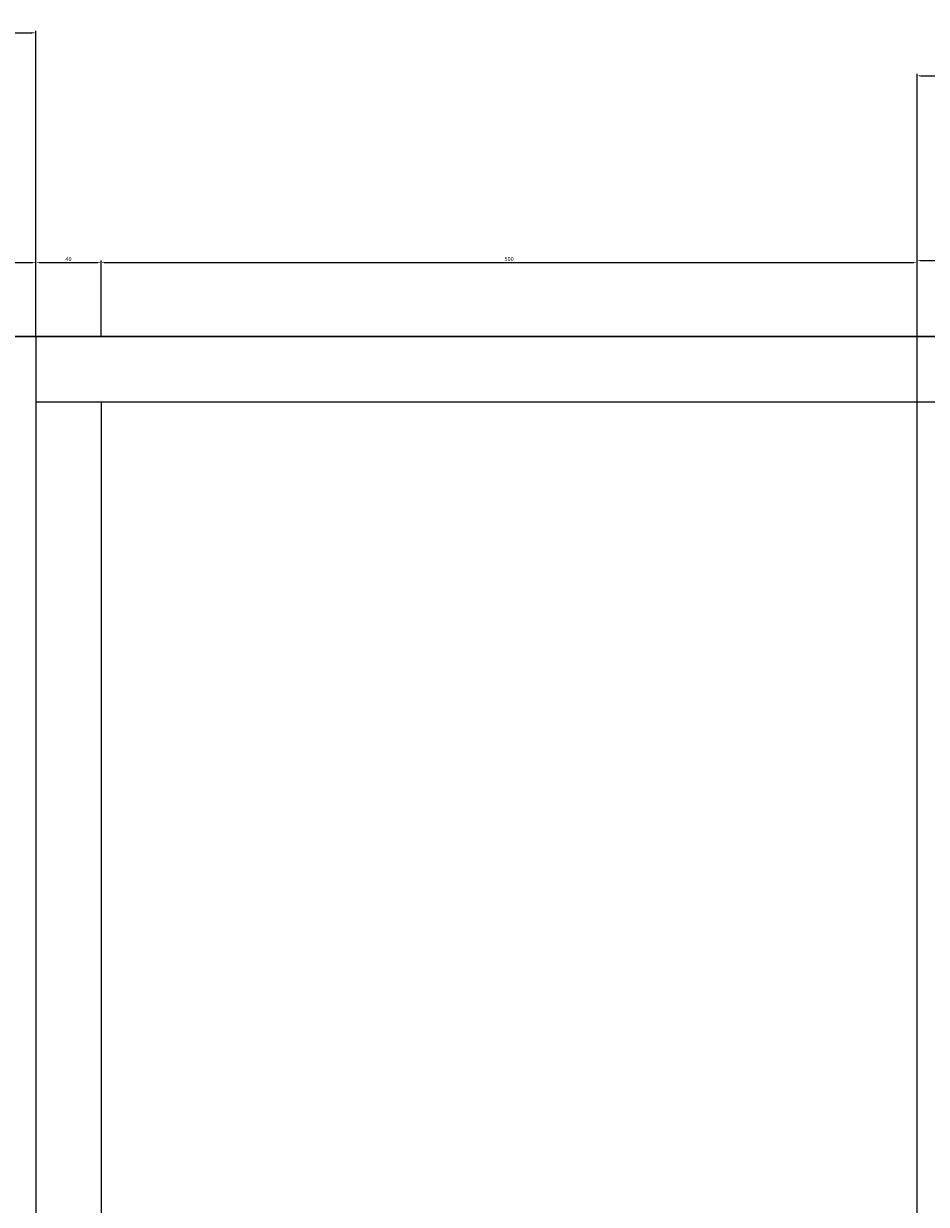
# Model space of a CAD drawing. Units: millimetres. Extents: x 2332 to 5836, y -853 to 2199.
# Tile 6 of 16: x 3088 to 3641, y 1476 to 2199. Entities that reach past the tile are written whole.
import ezdxf

# ---------------------------------------------------------------- set-up
doc = ezdxf.new("R2010")
doc.units = ezdxf.units.MM
doc.layers.get('0').update_dxf_attribs({"color": 8})
for name, color, linetype, lineweight in [('A-ANNO-DIMS', 2, 'Continuous', 18), ('A-WALL', 8, 'Continuous', 30), ('SHELF', 40, 'Continuous', 25)]:
    doc.layers.add(name, color=color, linetype=linetype, lineweight=lineweight)
doc.styles.get("Standard").update_dxf_attribs({"font": 'arial.ttf'})
doc.dimstyles.new('ISO-25', dxfattribs={"dimtxt": 2.5, "dimasz": 2.5, "dimexe": 1.25, "dimexo": 0.625, "dimtad": 1, "dimtxsty": 'Standard', "dimcen": 2.5, "dimadec": 0, "dimazin": 0, "dimtfac": 1, "dimtmove": 0, "dimatfit": 3, "dimfxl": 1, "dimarcsym": 0})

# ---------------------------------------------------------------- blocks, each defined once
blk = doc.blocks.new('*D1')
at = {"layer": 'A-ANNO-DIMS', "color": 0, "lineweight": -2, "transparency": 16777216}
for p, q in [((2745.04, 2008.43), (2745.04, 2054.25)), ((3095.04, 2008.43), (3095.04, 2054.25)), ((2747.54, 2053), (3092.54, 2053))]:
    blk.add_line(p, q, dxfattribs=at)
at = {"layer": 'A-ANNO-DIMS', "color": 0, "transparency": 16777216}
for points in [[(2747.54, 2053.41), (2747.54, 2052.58), (2745.04, 2053)], [(3092.54, 2053.41), (3092.54, 2052.58), (3095.04, 2053)]]:
    blk.add_solid(points, dxfattribs=at)
at = {"layer": 'Defpoints', "color": 0, "transparency": 16777216}
for p in [(3095.04, 2053), (2745.04, 2007.8), (3095.04, 2007.8)]:
    blk.add_point(p, dxfattribs=at)
at = {"layer": 'A-ANNO-DIMS', "color": 0, "transparency": 16777216, "insert": (2920.04, 2054.9), "char_height": 2.5, "attachment_point": 5}
blk.add_mtext('350', dxfattribs=at)
blk = doc.blocks.new('*D2')
at = {"layer": 'A-ANNO-DIMS', "color": 0, "lineweight": -2, "transparency": 16777216}
for p, q in [((3095.04, 2008.43), (3095.04, 2054.25)), ((3135.04, 2008.43), (3135.04, 2054.25)), ((3097.54, 2053), (3132.54, 2053))]:
    blk.add_line(p, q, dxfattribs=at)
at = {"layer": 'A-ANNO-DIMS', "color": 0, "transparency": 16777216}
for points in [[(3097.54, 2053.41), (3097.54, 2052.58), (3095.04, 2053)], [(3132.54, 2053.41), (3132.54, 2052.58), (3135.04, 2053)]]:
    blk.add_solid(points, dxfattribs=at)
at = {"layer": 'Defpoints', "color": 0, "transparency": 16777216}
for p in [(3135.04, 2053), (3095.04, 2007.8), (3135.04, 2007.8)]:
    blk.add_point(p, dxfattribs=at)
at = {"layer": 'A-ANNO-DIMS', "color": 0, "transparency": 16777216, "insert": (3115.04, 2054.9), "char_height": 2.5, "attachment_point": 5}
blk.add_mtext('40', dxfattribs=at)
blk = doc.blocks.new('*D3')
at = {"layer": 'A-ANNO-DIMS', "color": 0, "lineweight": -2, "transparency": 16777216}
for p, q in [((3135.04, 2008.43), (3135.04, 2054.25)), ((3635.04, 2008.43), (3635.04, 2054.25)), ((3137.54, 2053), (3632.54, 2053))]:
    blk.add_line(p, q, dxfattribs=at)
at = {"layer": 'A-ANNO-DIMS', "color": 0, "transparency": 16777216}
for points in [[(3137.54, 2053.41), (3137.54, 2052.58), (3135.04, 2053)], [(3632.54, 2053.41), (3632.54, 2052.58), (3635.04, 2053)]]:
    blk.add_solid(points, dxfattribs=at)
at = {"layer": 'Defpoints', "color": 0, "transparency": 16777216}
for p in [(3635.04, 2053), (3135.04, 2007.8), (3635.04, 2007.8)]:
    blk.add_point(p, dxfattribs=at)
at = {"layer": 'A-ANNO-DIMS', "color": 0, "transparency": 16777216, "insert": (3385.04, 2054.9), "char_height": 2.5, "attachment_point": 5}
blk.add_mtext('500', dxfattribs=at)
blk = doc.blocks.new('*D4')
at = {"layer": 'A-ANNO-DIMS', "color": 0, "lineweight": -2, "transparency": 16777216}
for p, q in [((3635.04, 2008.43), (3635.04, 2055.5)), ((3637.54, 2054.25), (4572.54, 2054.25)), ((4575.04, 2008.43), (4575.04, 2055.5))]:
    blk.add_line(p, q, dxfattribs=at)
at = {"layer": 'A-ANNO-DIMS', "color": 0, "transparency": 16777216}
for points in [[(3637.54, 2054.66), (3637.54, 2053.83), (3635.04, 2054.25)], [(4572.54, 2054.66), (4572.54, 2053.83), (4575.04, 2054.25)]]:
    blk.add_solid(points, dxfattribs=at)
at = {"layer": 'Defpoints', "color": 0, "transparency": 16777216}
for p in [(4575.04, 2054.25), (3635.04, 2007.8), (4575.04, 2007.8)]:
    blk.add_point(p, dxfattribs=at)
at = {"layer": 'A-ANNO-DIMS', "color": 0, "transparency": 16777216, "insert": (4105.04, 2056.15), "char_height": 2.5, "attachment_point": 5}
blk.add_mtext('940', dxfattribs=at)
blk = doc.blocks.new('CAB-END-STILE')
blk.add_line((113.09, 1240), (113.09, 0))
blk = doc.blocks.new('*D12')
at = {"layer": 'A-ANNO-DIMS', "color": 0, "lineweight": -2, "transparency": 16777216}
for p, q in [((2981.95, 2008.43), (2981.95, 2195.05)), ((2984.45, 2193.8), (3092.54, 2193.8)), ((3095.04, 2008.43), (3095.04, 2195.05))]:
    blk.add_line(p, q, dxfattribs=at)
at = {"layer": 'A-ANNO-DIMS', "color": 0, "transparency": 16777216}
for points in [[(2984.45, 2194.22), (2984.45, 2193.39), (2981.95, 2193.8)], [(3092.54, 2194.22), (3092.54, 2193.39), (3095.04, 2193.8)]]:
    blk.add_solid(points, dxfattribs=at)
at = {"layer": 'Defpoints', "color": 0, "transparency": 16777216}
for p in [(3095.04, 2193.8), (2981.95, 2007.8), (3095.04, 2007.8)]:
    blk.add_point(p, dxfattribs=at)
at = {"layer": 'A-ANNO-DIMS', "color": 0, "transparency": 16777216, "insert": (3038.49, 2195.71), "char_height": 2.5, "attachment_point": 5}
blk.add_mtext('113 TYP.', dxfattribs=at)
blk = doc.blocks.new('*D30')
at = {"layer": 'A-ANNO-DIMS', "color": 0, "lineweight": -2, "transparency": 16777216}
for p, q in [((3635.04, 1368.43), (3635.04, 2168.7)), ((3637.54, 2167.45), (4207.54, 2167.45)), ((4210.04, 1368.43), (4210.04, 2168.7))]:
    blk.add_line(p, q, dxfattribs=at)
at = {"layer": 'A-ANNO-DIMS', "color": 0, "transparency": 16777216}
for points in [[(3637.54, 2167.87), (3637.54, 2167.04), (3635.04, 2167.45)], [(4207.54, 2167.87), (4207.54, 2167.04), (4210.04, 2167.45)]]:
    blk.add_solid(points, dxfattribs=at)
at = {"layer": 'Defpoints', "color": 0, "transparency": 16777216}
for p in [(4210.04, 2167.45), (3635.04, 1367.8), (4210.04, 1367.8)]:
    blk.add_point(p, dxfattribs=at)
at = {"layer": 'A-ANNO-DIMS', "color": 0, "transparency": 16777216, "insert": (3922.54, 2169.35), "char_height": 2.5, "attachment_point": 5}
blk.add_mtext('575', dxfattribs=at)

msp = doc.modelspace()

# ---------------------------------------------------------------- linework, layer by layer
at = {"layer": 'A-WALL'}
for p, q in [((2745.04, 2007.803), (3095.04, 2007.803)), ((3095.04, 2007.803), (3135.04, 2007.803)), ((3135.04, 2007.803), (3635.04, 2007.803)), ((3635.04, 2007.803), (4575.04, 2007.803))]:
    msp.add_line(p, q, dxfattribs=at)
at = {"layer": 'SHELF'}
for p, q in [((3095.04, 1967.803), (4785.04, 1967.803)), ((3135.04, 1967.803), (3135.04, 767.803)), ((3635.04, 767.803), (3635.04, 1967.803))]:
    msp.add_line(p, q, dxfattribs=at)

# ---------------------------------------------------------------- block references
msp.add_blockref('CAB-END-STILE', (2981.95, 767.803), dxfattribs=at)

# ---------------------------------------------------------------- dimensions: what is measured, and where the dimension line sits
at = {"layer": 'A-ANNO-DIMS'}
dim = msp.add_linear_dim(base=(3095.04, 2193.803), p1=(2981.95, 2007.803), p2=(3095.04, 2007.803), text='<> TYP.', dimstyle='ISO-25', override={"dimdec": 0, "dimlfac": 1, "dimrnd": 0, "dimzin": 0, "dimdsep": 46, "dimlunit": 2}, dxfattribs=at)
dim.commit()
dim.dimension.update_dxf_attribs({"geometry": '*D12', "text_midpoint": (3038.495, 2195.706)})
for base, p1, p2, override, picture, middle in [((4210.04, 2167.453), (3635.04, 1367.803), (4210.04, 1367.803), {"dimdec": 0, "dimlfac": 1, "dimrnd": 0, "dimzin": 0, "dimdsep": 46, "dimlunit": 2}, '*D30', (3922.54, 2169.35)), ((3095.04, 2052.998), (2745.04, 2007.803), (3095.04, 2007.803), {"dimclrd": 0, "dimclre": 0, "dimclrt": 0}, '*D1', (2920.04, 2054.9)), ((3135.04, 2052.998), (3095.04, 2007.803), (3135.04, 2007.803), {"dimclrd": 0, "dimclre": 0, "dimclrt": 0}, '*D2', (3115.04, 2054.899)), ((3635.04, 2052.998), (3135.04, 2007.803), (3635.04, 2007.803), {"dimclrd": 0, "dimclre": 0, "dimclrt": 0}, '*D3', (3385.04, 2054.899)), ((4575.04, 2054.248), (3635.04, 2007.803), (4575.04, 2007.803), {"dimclrd": 0, "dimclre": 0, "dimclrt": 0}, '*D4', (4105.04, 2056.149))]:
    dim = msp.add_linear_dim(base=base, p1=p1, p2=p2, dimstyle='ISO-25', override=override, dxfattribs=at)
    dim.commit()
    dim.dimension.update_dxf_attribs({"geometry": picture, "text_midpoint": middle})

doc.saveas('drawing.dxf')
